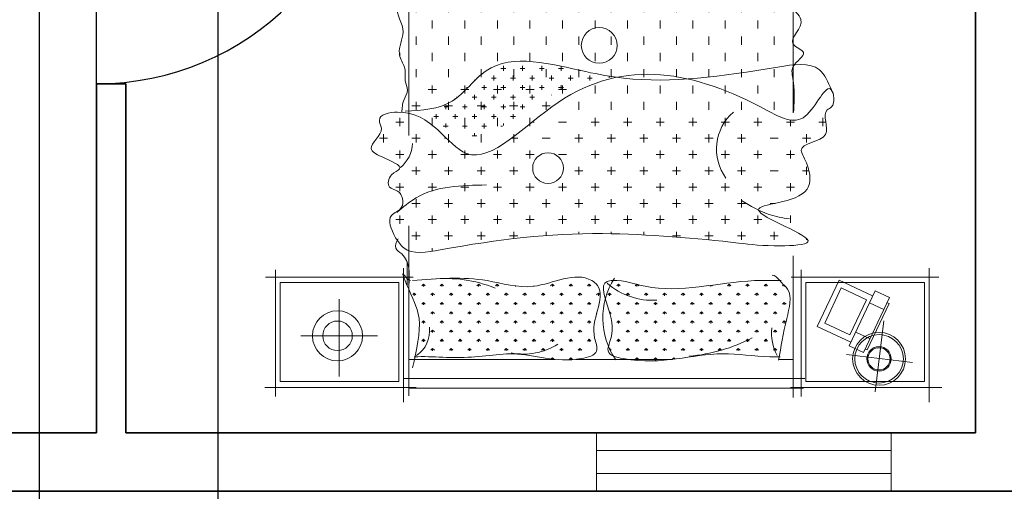
# Model space of a CAD drawing. Units: inches. Extents: x -26 to 575, y -18 to 513.
# Tile 3 of 28: x 122 to 274, y 119 to 191. Entities that reach past the tile are written whole.
import ezdxf

# ---------------------------------------------------------------- set-up
doc = ezdxf.new("R2010")
doc.units = ezdxf.units.IN
doc.header["$MEASUREMENT"] = 0
for name, color, linetype, lineweight in [('A-ANNO-DIMS', 2, 'Continuous', 18), ('A-DOOR', 3, 'Continuous', 25), ('A-GLAZ', 4, 'Continuous', 18), ('A-WALL', 7, 'Continuous', 35), ('Furniture', 8, 'Continuous', 15)]:
    doc.layers.add(name, color=color, linetype=linetype, lineweight=lineweight)
doc.styles.get("Standard").update_dxf_attribs({"font": 'arial.ttf', "height": 6})
doc.dimstyles.get("Standard").update_dxf_attribs({"dimtxt": 6, "dimasz": 0.18, "dimexe": 0.18, "dimexo": 0.0625, "dimgap": 0.09, "dimtad": 0, "dimtih": 1, "dimtoh": 1, "dimzin": 0, "dimdsep": 46, "dimlunit": 3, "dimtxsty": 'Standard', "dimcen": 0.09, "dimadec": 0, "dimazin": 0, "dimtfac": 1, "dimtofl": 0, "dimtmove": 0, "dimatfit": 3, "dimfxl": 1, "dimtolj": 1, "dimtzin": 0, "dimarcsym": 0})

# ---------------------------------------------------------------- blocks, each defined once
blk = doc.blocks.new('BED-DOUBLE-WITH-NIGHTSTANDS')
for p, q in [((1.93, 83.36), (1.93, 62.76)), ((82.67, 83.36), (82.67, 62.76)), ((10.27, 81.76), (8.94, 70.83)), ((21.61, 63.03), (21.61, 82.46)), ((22.83, 60.83), (22.83, 82.62)), ((81.88, 82.34), (81.88, 56.23)), ((102.35, 63.03), (102.35, 82.46)), ((23.23, 81.08), (0, 81.08)), ((20.89, 80.15), (2.67, 80.15)), ((2.67, 80.15), (2.67, 64.97)), ((20.89, 64.97), (20.89, 80.15)), ((21.24, 81.17), (81.88, 81.17)), ((103.97, 81.08), (80.74, 81.08)), ((101.63, 80.15), (83.41, 80.15)), ((83.41, 80.15), (83.41, 64.97)), ((101.63, 64.97), (101.63, 80.15)), ((82.67, 79.72), (21.06, 79.72)), ((92.57, 79.4), (92.57, 67.51)), ((14.67, 76.01), (4.51, 77.26)), ((8.06, 67.24), (12.03, 75.72)), ((12.03, 75.72), (14.23, 74.69)), ((25.06, 76.76), (22.83, 76.76)), ((41.17, 76.51), (40.96, 76.72)), ((41.17, 76.51), (41.43, 76.77)), ((41.17, 76.51), (41.17, 76.74)), ((56.23, 76.76), (41.36, 76.76)), ((44, 76.51), (43.73, 76.77)), ((44, 76.51), (44, 76.88)), ((44, 76.51), (44.26, 76.77)), ((46.83, 76.51), (46.56, 76.77)), ((46.83, 76.51), (46.83, 76.88)), ((46.83, 76.51), (47.09, 76.77)), ((57, 76.51), (56.74, 76.77)), ((57, 76.51), (57, 76.83)), ((57, 76.51), (57.27, 76.77)), ((81.88, 76.76), (59.39, 76.76)), ((59.83, 76.51), (59.59, 76.74)), ((59.83, 76.51), (59.83, 76.72)), ((59.83, 76.51), (60.02, 76.69)), ((11.46, 75.32), (8.12, 68.2)), ((14.23, 74.69), (10.26, 66.21)), ((11.77, 75.18), (11.46, 75.32)), ((19.14, 71.73), (13.98, 74.14)), ((25.61, 75.09), (25.35, 75.36)), ((25.61, 75.09), (25.61, 75.47)), ((25.61, 75.09), (25.88, 75.36)), ((28.44, 75.09), (28.18, 75.36)), ((28.44, 75.09), (28.44, 75.47)), ((28.44, 75.09), (28.71, 75.36)), ((31.27, 75.09), (31, 75.36)), ((31.27, 75.09), (31.27, 75.47)), ((31.27, 75.09), (31.53, 75.36)), ((34.1, 75.09), (33.83, 75.36)), ((34.1, 75.09), (34.1, 75.47)), ((34.1, 75.09), (34.36, 75.36)), ((36.93, 75.09), (36.66, 75.36)), ((36.93, 75.09), (36.93, 75.47)), ((36.93, 75.09), (37.19, 75.36)), ((39.75, 75.09), (39.49, 75.36)), ((39.75, 75.09), (39.75, 75.47)), ((39.75, 75.09), (40.02, 75.36)), ((42.58, 75.09), (42.32, 75.36)), ((42.58, 75.09), (42.58, 75.47)), ((42.58, 75.09), (42.85, 75.36)), ((45.41, 75.09), (45.15, 75.36)), ((45.41, 75.09), (45.41, 75.47)), ((45.41, 75.09), (45.68, 75.36)), ((48.24, 75.09), (47.97, 75.36)), ((48.24, 75.09), (48.24, 75.47)), ((48.24, 75.09), (48.5, 75.36)), ((51.07, 75.09), (50.8, 75.36)), ((51.07, 75.09), (51.07, 75.1)), ((51.07, 75.09), (51.07, 75.1)), ((53, 75.34), (53.03, 75.36)), ((55.59, 75.09), (55.32, 75.36)), ((55.59, 75.09), (55.59, 75.47)), ((55.59, 75.09), (55.85, 75.36)), ((58.42, 75.09), (58.15, 75.36)), ((58.42, 75.09), (58.42, 75.47)), ((58.42, 75.09), (58.68, 75.36)), ((61.25, 75.09), (60.98, 75.36)), ((61.25, 75.09), (61.25, 75.47)), ((61.25, 75.09), (61.51, 75.36)), ((64.07, 75.09), (63.81, 75.36)), ((64.07, 75.09), (64.07, 75.47)), ((64.07, 75.09), (64.34, 75.36)), ((66.9, 75.09), (66.64, 75.36)), ((66.9, 75.09), (66.9, 75.47)), ((66.9, 75.09), (67.17, 75.36)), ((69.73, 75.09), (69.47, 75.36)), ((69.73, 75.09), (69.73, 75.47)), ((69.73, 75.09), (70, 75.36)), ((72.56, 75.09), (72.29, 75.36)), ((72.56, 75.09), (72.56, 75.47)), ((72.56, 75.09), (72.82, 75.36)), ((75.39, 75.09), (75.12, 75.36)), ((75.39, 75.09), (75.39, 75.47)), ((75.39, 75.09), (75.65, 75.36)), ((78.22, 75.09), (77.95, 75.36)), ((78.22, 75.09), (78.22, 75.47)), ((78.22, 75.09), (78.48, 75.36)), ((13.24, 72.57), (11.03, 73.6)), ((14.13, 73), (11.6, 67.59)), ((17.98, 71.2), (14.13, 73)), ((25.61, 72.26), (25.61, 72.64)), ((27.03, 73.68), (26.76, 73.94)), ((27.03, 73.68), (27.03, 74.05)), ((27.03, 73.68), (27.29, 73.94)), ((28.44, 72.26), (28.44, 72.64)), ((29.85, 73.68), (29.59, 73.94)), ((29.85, 73.68), (30.12, 73.94)), ((29.86, 73.68), (29.86, 74.05)), ((31.27, 72.26), (31.27, 72.64)), ((32.68, 73.68), (32.42, 73.94)), ((32.68, 73.68), (32.68, 74.05)), ((32.68, 73.68), (32.95, 73.94)), ((34.1, 72.26), (34.1, 72.64)), ((35.51, 73.68), (35.25, 73.94)), ((35.51, 73.68), (35.51, 74.05)), ((35.51, 73.68), (35.78, 73.94)), ((36.93, 72.26), (36.93, 72.64)), ((38.34, 73.68), (38.07, 73.94)), ((38.34, 73.68), (38.34, 74.05)), ((38.34, 73.68), (38.61, 73.94)), ((39.75, 72.26), (39.75, 72.64)), ((41.17, 73.68), (40.9, 73.94)), ((41.17, 73.68), (41.17, 74.05)), ((41.17, 73.68), (41.43, 73.94)), ((42.58, 72.26), (42.58, 72.64)), ((44, 73.68), (43.73, 73.94)), ((44, 73.68), (44, 74.05)), ((44, 73.68), (44.26, 73.94)), ((45.41, 72.26), (45.41, 72.64)), ((46.83, 73.68), (46.56, 73.94)), ((46.83, 73.68), (46.83, 74.05)), ((46.83, 73.68), (47.09, 73.94)), ((48.24, 72.26), (48.24, 72.64)), ((49.65, 73.68), (49.39, 73.94)), ((49.65, 73.68), (49.65, 74.05)), ((49.65, 73.68), (49.92, 73.94)), ((54.17, 73.68), (53.91, 73.94)), ((54.17, 73.68), (54.17, 74.05)), ((54.17, 73.68), (54.44, 73.94)), ((55.59, 72.26), (55.59, 72.64)), ((57, 73.68), (56.74, 73.94)), ((57, 73.68), (57, 74.05)), ((57, 73.68), (57.27, 73.94)), ((58.42, 72.26), (58.42, 72.64)), ((59.83, 73.68), (59.57, 73.94)), ((59.83, 73.68), (59.83, 74.05)), ((59.83, 73.68), (60.1, 73.94)), ((61.25, 72.26), (61.25, 72.64)), ((62.66, 73.68), (62.39, 73.94)), ((62.66, 73.68), (62.66, 74.05)), ((62.66, 73.68), (62.92, 73.94)), ((64.07, 72.26), (64.07, 72.64)), ((65.49, 73.68), (65.22, 73.94)), ((65.49, 73.68), (65.49, 74.05)), ((65.49, 73.68), (65.75, 73.94)), ((66.9, 72.26), (66.9, 72.64)), ((68.32, 73.68), (68.05, 73.94)), ((68.32, 73.68), (68.32, 74.05)), ((68.32, 73.68), (68.58, 73.94)), ((69.73, 72.26), (69.73, 72.64)), ((71.14, 73.68), (70.88, 73.94)), ((71.14, 73.68), (71.41, 73.94)), ((71.15, 73.68), (71.15, 74.05)), ((72.56, 72.26), (72.56, 72.64)), ((73.97, 73.68), (73.71, 73.94)), ((73.97, 73.68), (73.97, 74.05)), ((73.97, 73.68), (74.24, 73.94)), ((75.39, 72.26), (75.39, 72.64)), ((76.8, 73.68), (76.54, 73.94)), ((76.8, 73.68), (76.8, 74.05)), ((76.8, 73.68), (77.07, 73.94)), ((78.22, 72.26), (78.22, 72.64)), ((79.63, 73.68), (79.36, 73.94)), ((79.63, 73.68), (79.63, 74.05)), ((79.63, 73.68), (79.9, 73.94)), ((98.47, 73.14), (86.67, 73.14)), ((15.45, 65.79), (17.98, 71.2)), ((15.8, 64.6), (19.14, 71.73)), ((24.2, 70.85), (23.97, 71.08)), ((24.2, 70.85), (24.2, 71.23)), ((24.2, 70.85), (24.46, 71.12)), ((25.61, 72.26), (25.35, 72.53)), ((25.61, 72.26), (25.88, 72.53)), ((27.03, 70.85), (26.76, 71.12)), ((27.03, 70.85), (27.03, 71.23)), ((27.03, 70.85), (27.29, 71.12)), ((28.44, 72.26), (28.18, 72.53)), ((28.44, 72.26), (28.71, 72.53)), ((29.85, 70.85), (29.59, 71.12)), ((29.85, 70.85), (30.12, 71.12)), ((29.86, 70.85), (29.86, 71.23)), ((31.27, 72.26), (31, 72.53)), ((31.27, 72.26), (31.53, 72.53)), ((32.68, 70.85), (32.42, 71.12)), ((32.68, 70.85), (32.68, 71.23)), ((32.68, 70.85), (32.95, 71.12)), ((34.1, 72.26), (33.83, 72.53)), ((34.1, 72.26), (34.36, 72.53)), ((35.51, 70.85), (35.25, 71.12)), ((35.51, 70.85), (35.51, 71.23)), ((35.51, 70.85), (35.78, 71.12)), ((36.93, 72.26), (36.66, 72.53)), ((36.93, 72.26), (37.19, 72.53)), ((38.34, 70.85), (38.07, 71.12)), ((38.34, 70.85), (38.34, 71.23)), ((38.34, 70.85), (38.61, 71.12)), ((39.75, 72.26), (39.49, 72.53)), ((39.75, 72.26), (40.02, 72.53)), ((41.17, 70.85), (40.9, 71.12)), ((41.17, 70.85), (41.17, 71.23)), ((41.17, 70.85), (41.43, 71.12)), ((42.58, 72.26), (42.32, 72.53)), ((42.58, 72.26), (42.85, 72.53)), ((44, 70.85), (43.73, 71.12)), ((44, 70.85), (44, 71.23)), ((44, 70.85), (44.26, 71.12)), ((45.41, 72.26), (45.15, 72.53)), ((45.41, 72.26), (45.68, 72.53)), ((46.83, 70.85), (46.56, 71.12)), ((46.83, 70.85), (46.83, 71.23)), ((46.83, 70.85), (47.09, 71.12)), ((48.24, 72.26), (47.97, 72.53)), ((48.24, 72.26), (48.5, 72.53)), ((49.65, 70.85), (49.39, 71.12)), ((49.65, 70.85), (49.65, 71.23)), ((49.65, 70.85), (49.92, 71.12)), ((54.17, 70.85), (53.91, 71.12)), ((54.17, 70.85), (54.17, 71.23)), ((54.17, 70.85), (54.44, 71.12)), ((55.59, 72.26), (55.32, 72.53)), ((55.59, 72.26), (55.85, 72.53)), ((57, 70.85), (56.74, 71.12)), ((57, 70.85), (57, 71.23)), ((57, 70.85), (57.27, 71.12)), ((58.42, 72.26), (58.15, 72.53)), ((58.42, 72.26), (58.68, 72.53)), ((59.83, 70.85), (59.57, 71.12)), ((59.83, 70.85), (59.83, 71.23)), ((59.83, 70.85), (60.1, 71.12)), ((61.25, 72.26), (60.98, 72.53)), ((61.25, 72.26), (61.51, 72.53)), ((62.66, 70.85), (62.39, 71.12)), ((62.66, 70.85), (62.66, 71.23)), ((62.66, 70.85), (62.92, 71.12)), ((64.07, 72.26), (63.81, 72.53)), ((64.07, 72.26), (64.34, 72.53)), ((65.49, 70.85), (65.22, 71.12)), ((65.49, 70.85), (65.49, 71.23)), ((65.49, 70.85), (65.75, 71.12)), ((66.9, 72.26), (66.64, 72.53)), ((66.9, 72.26), (67.17, 72.53)), ((68.32, 70.85), (68.05, 71.12)), ((68.32, 70.85), (68.32, 71.23)), ((68.32, 70.85), (68.58, 71.12)), ((69.73, 72.26), (69.47, 72.53)), ((69.73, 72.26), (70, 72.53)), ((71.14, 70.85), (70.88, 71.12)), ((71.14, 70.85), (71.41, 71.12)), ((71.15, 70.85), (71.15, 71.23)), ((72.56, 72.26), (72.29, 72.53)), ((72.56, 72.26), (72.82, 72.53)), ((73.97, 70.85), (73.71, 71.12)), ((73.97, 70.85), (73.97, 71.23)), ((73.97, 70.85), (74.24, 71.12)), ((75.39, 72.26), (75.12, 72.53)), ((75.39, 72.26), (75.65, 72.53)), ((76.8, 70.85), (76.54, 71.12)), ((76.8, 70.85), (76.8, 71.23)), ((76.8, 70.85), (77.07, 71.12)), ((78.22, 72.26), (77.95, 72.53)), ((78.22, 72.26), (78.48, 72.53)), ((79.63, 70.85), (79.36, 71.12)), ((79.63, 70.85), (79.63, 71.23)), ((79.63, 70.85), (79.9, 71.12)), ((25.61, 69.44), (25.35, 69.7)), ((25.61, 69.44), (25.61, 69.81)), ((25.61, 69.44), (25.88, 69.7)), ((28.44, 69.44), (28.18, 69.7)), ((28.44, 69.44), (28.44, 69.81)), ((28.44, 69.44), (28.71, 69.7)), ((31.27, 69.44), (31, 69.7)), ((31.27, 69.44), (31.27, 69.81)), ((31.27, 69.44), (31.53, 69.7)), ((34.1, 69.44), (33.83, 69.7)), ((34.1, 69.44), (34.1, 69.81)), ((34.1, 69.44), (34.36, 69.7)), ((36.93, 69.44), (36.66, 69.7)), ((36.93, 69.44), (36.93, 69.81)), ((36.93, 69.44), (37.19, 69.7)), ((39.75, 69.44), (39.49, 69.7)), ((39.75, 69.44), (39.75, 69.81)), ((39.75, 69.44), (40.02, 69.7)), ((42.58, 69.44), (42.32, 69.7)), ((42.58, 69.44), (42.58, 69.81)), ((42.58, 69.44), (42.85, 69.7)), ((45.41, 69.44), (45.15, 69.7)), ((45.41, 69.44), (45.41, 69.81)), ((45.41, 69.44), (45.68, 69.7)), ((48.24, 69.44), (47.97, 69.7)), ((48.24, 69.44), (48.24, 69.81)), ((48.24, 69.44), (48.5, 69.7)), ((51.05, 69.45), (50.8, 69.7)), ((53.01, 69.68), (53.03, 69.7)), ((55.59, 69.44), (55.32, 69.7)), ((55.59, 69.44), (55.59, 69.81)), ((55.59, 69.44), (55.85, 69.7)), ((58.42, 69.44), (58.15, 69.7)), ((58.42, 69.44), (58.42, 69.81)), ((58.42, 69.44), (58.68, 69.7)), ((61.25, 69.44), (60.98, 69.7)), ((61.25, 69.44), (61.25, 69.81)), ((61.25, 69.44), (61.51, 69.7)), ((64.07, 69.44), (63.81, 69.7)), ((64.07, 69.44), (64.07, 69.81)), ((64.07, 69.44), (64.34, 69.7)), ((66.9, 69.44), (66.64, 69.7)), ((66.9, 69.44), (66.9, 69.81)), ((66.9, 69.44), (67.17, 69.7)), ((69.73, 69.44), (69.47, 69.7)), ((69.73, 69.44), (69.73, 69.81)), ((69.73, 69.44), (70, 69.7)), ((72.56, 69.44), (72.29, 69.7)), ((72.56, 69.44), (72.56, 69.81)), ((72.56, 69.44), (72.82, 69.7)), ((75.39, 69.44), (75.12, 69.7)), ((75.39, 69.44), (75.39, 69.81)), ((75.39, 69.44), (75.65, 69.7)), ((78.22, 69.44), (77.95, 69.7)), ((78.22, 69.44), (78.22, 69.81)), ((78.22, 69.44), (78.48, 69.7)), ((8.12, 68.2), (8.43, 68.05)), ((11.14, 68.07), (8.93, 69.1)), ((24.2, 68.02), (23.93, 68.29)), ((24.2, 68.02), (24.2, 68.4)), ((24.2, 68.02), (24.46, 68.29)), ((27.03, 68.02), (26.76, 68.29)), ((27.03, 68.02), (27.03, 68.4)), ((27.03, 68.02), (27.29, 68.29)), ((29.85, 68.02), (29.59, 68.29)), ((29.85, 68.02), (30.12, 68.29)), ((29.86, 68.02), (29.86, 68.4)), ((32.68, 68.02), (32.42, 68.29)), ((32.68, 68.02), (32.68, 68.4)), ((32.68, 68.02), (32.95, 68.29)), ((35.51, 68.02), (35.25, 68.29)), ((35.51, 68.02), (35.51, 68.4)), ((35.51, 68.02), (35.78, 68.29)), ((38.34, 68.02), (38.07, 68.29)), ((38.34, 68.02), (38.34, 68.4)), ((38.34, 68.02), (38.61, 68.29)), ((41.17, 68.02), (40.9, 68.29)), ((41.17, 68.02), (41.17, 68.4)), ((41.17, 68.02), (41.43, 68.29)), ((44, 68.02), (43.73, 68.29)), ((44, 68.02), (44, 68.4)), ((44, 68.02), (44.26, 68.29)), ((46.83, 68.02), (46.56, 68.29)), ((46.83, 68.02), (46.83, 68.4)), ((46.83, 68.02), (47.09, 68.29)), ((49.65, 68.02), (49.39, 68.29)), ((49.65, 68.02), (49.65, 68.4)), ((49.65, 68.02), (49.92, 68.29)), ((54.17, 68.02), (53.91, 68.29)), ((54.17, 68.02), (54.17, 68.4)), ((54.17, 68.02), (54.44, 68.29)), ((57, 68.02), (56.74, 68.29)), ((57, 68.02), (57, 68.4)), ((57, 68.02), (57.27, 68.29)), ((59.83, 68.02), (59.57, 68.29)), ((59.83, 68.02), (59.83, 68.4)), ((59.83, 68.02), (60.1, 68.29)), ((62.66, 68.02), (62.39, 68.29)), ((62.66, 68.02), (62.66, 68.4)), ((62.66, 68.02), (62.92, 68.29)), ((65.49, 68.02), (65.22, 68.29)), ((65.49, 68.02), (65.49, 68.4)), ((65.49, 68.02), (65.75, 68.29)), ((68.32, 68.02), (68.05, 68.29)), ((68.32, 68.02), (68.32, 68.4)), ((68.32, 68.02), (68.58, 68.29)), ((71.14, 68.02), (70.88, 68.29)), ((71.14, 68.02), (71.41, 68.29)), ((71.15, 68.02), (71.15, 68.4)), ((73.97, 68.02), (73.71, 68.29)), ((73.97, 68.02), (73.97, 68.4)), ((73.97, 68.02), (74.24, 68.29)), ((76.8, 68.02), (76.54, 68.29)), ((76.8, 68.02), (76.8, 68.4)), ((76.8, 68.02), (77.07, 68.29)), ((79.63, 68.02), (79.36, 68.29)), ((79.63, 68.02), (79.63, 68.4)), ((79.63, 68.02), (79.9, 68.29)), ((10.26, 66.21), (8.06, 67.24)), ((10.64, 67.02), (15.8, 64.6)), ((11.6, 67.59), (15.45, 65.79)), ((25.61, 66.61), (25.35, 66.87)), ((25.61, 66.61), (25.61, 66.98)), ((25.61, 66.61), (25.88, 66.87)), ((28.44, 66.61), (28.18, 66.87)), ((28.44, 66.61), (28.44, 66.98)), ((28.44, 66.61), (28.71, 66.87)), ((31.27, 66.61), (31, 66.87)), ((31.27, 66.61), (31.27, 66.98)), ((31.27, 66.61), (31.53, 66.87)), ((34.1, 66.61), (33.83, 66.87)), ((34.1, 66.61), (34.1, 66.98)), ((34.1, 66.61), (34.36, 66.87)), ((36.93, 66.61), (36.66, 66.87)), ((36.93, 66.61), (36.93, 66.98)), ((36.93, 66.61), (37.19, 66.87)), ((39.75, 66.61), (39.49, 66.87)), ((39.75, 66.61), (39.75, 66.98)), ((39.75, 66.61), (40.02, 66.87)), ((42.58, 66.61), (42.32, 66.87)), ((42.58, 66.61), (42.58, 66.98)), ((42.58, 66.61), (42.85, 66.87)), ((45.41, 66.61), (45.15, 66.87)), ((45.41, 66.61), (45.41, 66.98)), ((45.41, 66.61), (45.68, 66.87)), ((48.24, 66.61), (47.97, 66.87)), ((48.24, 66.61), (48.24, 66.98)), ((48.24, 66.61), (48.5, 66.87)), ((51.07, 66.61), (50.8, 66.87)), ((51.07, 66.61), (51.07, 66.98)), ((51.07, 66.61), (51.33, 66.87)), ((52.76, 66.61), (52.49, 66.87)), ((52.76, 66.61), (52.76, 66.98)), ((52.76, 66.61), (53.03, 66.87)), ((55.59, 66.61), (55.32, 66.87)), ((55.59, 66.61), (55.59, 66.98)), ((55.59, 66.61), (55.85, 66.87)), ((58.42, 66.61), (58.15, 66.87)), ((58.42, 66.61), (58.42, 66.98)), ((58.42, 66.61), (58.68, 66.87)), ((61.25, 66.61), (60.98, 66.87)), ((61.25, 66.61), (61.25, 66.98)), ((61.25, 66.61), (61.51, 66.87)), ((64.07, 66.61), (63.81, 66.87)), ((64.07, 66.61), (64.07, 66.98)), ((64.07, 66.61), (64.34, 66.87)), ((66.9, 66.61), (66.64, 66.87)), ((66.9, 66.61), (66.9, 66.98)), ((66.9, 66.61), (67.17, 66.87)), ((69.73, 66.61), (69.47, 66.87)), ((69.73, 66.61), (69.73, 66.98)), ((69.73, 66.61), (70, 66.87)), ((72.56, 66.61), (72.29, 66.87)), ((72.56, 66.61), (72.56, 66.98)), ((72.56, 66.61), (72.82, 66.87)), ((75.39, 66.61), (75.12, 66.87)), ((75.39, 66.61), (75.39, 66.98)), ((75.39, 66.61), (75.65, 66.87)), ((78.22, 66.61), (77.95, 66.87)), ((78.22, 66.61), (78.22, 66.98)), ((78.22, 66.61), (78.48, 66.87)), ((81.04, 66.61), (80.78, 66.87)), ((81.04, 66.61), (81.04, 66.98)), ((81.04, 66.61), (81.25, 66.82)), ((24.2, 65.39), (24.2, 65.57)), ((24.29, 65.29), (24.46, 65.46)), ((27.03, 65.19), (26.76, 65.46)), ((27.03, 65.19), (27.03, 65.57)), ((27.03, 65.19), (27.29, 65.46)), ((29.85, 65.19), (29.59, 65.46)), ((29.85, 65.19), (30.12, 65.46)), ((29.86, 65.19), (29.86, 65.57)), ((32.68, 65.19), (32.42, 65.46)), ((32.68, 65.19), (32.68, 65.57)), ((32.68, 65.19), (32.95, 65.46)), ((35.33, 65.37), (35.25, 65.46)), ((35.51, 65.39), (35.51, 65.57)), ((35.74, 65.42), (35.78, 65.46)), ((46.77, 65.25), (46.56, 65.46)), ((46.83, 65.23), (46.83, 65.57)), ((46.86, 65.22), (47.09, 65.46)), ((49.65, 65.19), (49.39, 65.46)), ((49.65, 65.19), (49.65, 65.57)), ((49.65, 65.19), (49.92, 65.46)), ((54.17, 65.19), (53.91, 65.46)), ((54.17, 65.19), (54.17, 65.57)), ((54.17, 65.19), (54.44, 65.46)), ((57, 65.19), (56.74, 65.46)), ((57, 65.19), (57, 65.57)), ((57, 65.19), (57.27, 65.46)), ((59.83, 65.19), (59.57, 65.46)), ((59.83, 65.19), (59.83, 65.57)), ((59.83, 65.19), (60.1, 65.46)), ((62.66, 65.52), (62.66, 65.57)), ((65.49, 65.48), (65.49, 65.57)), ((65.74, 65.45), (65.75, 65.46)), ((68.32, 65.19), (68.05, 65.46)), ((68.32, 65.19), (68.32, 65.57)), ((68.32, 65.19), (68.58, 65.46)), ((71.14, 65.19), (70.88, 65.46)), ((71.14, 65.19), (71.41, 65.46)), ((71.15, 65.19), (71.15, 65.57)), ((73.97, 65.19), (73.71, 65.46)), ((73.97, 65.19), (73.97, 65.57)), ((73.97, 65.19), (74.24, 65.46)), ((76.8, 65.19), (76.54, 65.46)), ((76.8, 65.19), (76.8, 65.57)), ((76.8, 65.19), (77.07, 65.46)), ((79.63, 65.19), (79.36, 65.46)), ((79.63, 65.19), (79.63, 65.57)), ((79.63, 65.19), (79.9, 65.46)), ((82.15, 61.74), (82.15, 65.42)), ((0.45, 64.15), (23.14, 64.15)), ((2.67, 64.97), (20.89, 64.97)), ((55.59, 64.12), (55.59, 64.15)), ((81.19, 64.15), (103.88, 64.15)), ((83.41, 64.97), (101.63, 64.97)), ((78.27, 59.67), (78.27, 60.15)), ((20.77, 58.21), (20.77, 58.42)), ((21.39, 57.79), (21.31, 57.79)), ((26.39, 57.79), (25.14, 57.79)), ((25.77, 57.17), (25.77, 58.42)), ((31.39, 57.79), (30.14, 57.79)), ((30.77, 57.17), (30.77, 58.42)), ((36.39, 57.79), (35.14, 57.79)), ((35.77, 57.17), (35.77, 58.41)), ((41.39, 57.79), (40.14, 57.79)), ((40.77, 57.17), (40.77, 57.97)), ((45.77, 57.17), (45.77, 57.64)), ((55.77, 57.17), (55.77, 57.48)), ((60.77, 57.17), (60.77, 57.74)), ((66.39, 57.79), (65.14, 57.79)), ((65.77, 57.17), (65.77, 58.21)), ((71.39, 57.79), (70.14, 57.79)), ((70.77, 57.17), (70.77, 58.42)), ((76.39, 57.79), (75.14, 57.79)), ((75.77, 57.17), (75.77, 58.42)), ((81.39, 57.79), (80.14, 57.79)), ((80.77, 57.17), (80.77, 58.42)), ((50.77, 57.17), (50.77, 57.46)), ((23.27, 54.64), (23.27, 55.76)), ((28.89, 55.29), (27.64, 55.29)), ((28.27, 54.67), (28.27, 55.92)), ((33.89, 55.29), (32.64, 55.29)), ((33.27, 54.67), (33.27, 55.92)), ((38.89, 55.29), (37.64, 55.29)), ((38.27, 54.67), (38.27, 55.92)), ((43.89, 55.29), (42.64, 55.29)), ((43.27, 54.67), (43.27, 55.92)), ((48.89, 55.29), (47.64, 55.29)), ((48.27, 54.67), (48.27, 55.92)), ((53.89, 55.29), (52.64, 55.29)), ((53.27, 54.67), (53.27, 55.92)), ((58.89, 55.29), (57.64, 55.29)), ((58.27, 54.67), (58.27, 55.92)), ((63.89, 55.29), (62.64, 55.29)), ((63.27, 54.67), (63.27, 55.92)), ((68.89, 55.29), (67.64, 55.29)), ((68.27, 54.67), (68.27, 55.92)), ((73.89, 55.29), (72.64, 55.29)), ((73.27, 54.67), (73.27, 55.92)), ((78.89, 55.29), (77.64, 55.29)), ((78.27, 54.67), (78.27, 55.92)), ((83.89, 55.29), (82.64, 55.29)), ((83.27, 54.67), (83.27, 55.92)), ((30.77, 52.17), (30.77, 53.42)), ((35.77, 52.17), (35.77, 53.42)), ((40.77, 52.17), (40.77, 53.42)), ((45.77, 52.17), (45.77, 53.42)), ((50.77, 52.17), (50.77, 53.42)), ((55.77, 52.17), (55.77, 53.42)), ((60.77, 52.17), (60.77, 53.42)), ((65.77, 52.17), (65.77, 53.42)), ((70.77, 52.17), (70.77, 53.42)), ((75.77, 52.17), (75.77, 53.42)), ((80.77, 52.17), (80.77, 53.42)), ((26.39, 52.79), (25.62, 52.79)), ((31.39, 52.79), (30.14, 52.79)), ((36.39, 52.79), (35.14, 52.79)), ((41.39, 52.79), (40.14, 52.79)), ((46.39, 52.79), (45.14, 52.79)), ((51.39, 52.79), (50.14, 52.79)), ((56.39, 52.79), (55.14, 52.79)), ((61.39, 52.79), (60.14, 52.79)), ((66.39, 52.79), (65.14, 52.79)), ((71.39, 52.79), (70.14, 52.79)), ((76.39, 52.79), (75.14, 52.79)), ((81.39, 52.79), (80.14, 52.79)), ((23.89, 50.29), (22.64, 50.29)), ((23.27, 49.67), (23.27, 50.92)), ((28.89, 50.29), (27.64, 50.29)), ((28.27, 49.67), (28.27, 50.92)), ((33.89, 50.29), (32.64, 50.29)), ((33.27, 49.67), (33.27, 50.92)), ((38.89, 50.29), (37.64, 50.29)), ((38.27, 49.67), (38.27, 50.92)), ((43.89, 50.29), (42.64, 50.29)), ((43.27, 49.67), (43.27, 50.92)), ((48.89, 50.29), (47.64, 50.29)), ((48.27, 49.67), (48.27, 50.92)), ((53.89, 50.29), (52.64, 50.29)), ((53.27, 49.67), (53.27, 50.92)), ((58.89, 50.29), (57.64, 50.29)), ((58.27, 49.67), (58.27, 50.92)), ((63.89, 50.29), (62.64, 50.29)), ((63.27, 49.67), (63.27, 50.92)), ((68.89, 50.29), (67.64, 50.29)), ((68.27, 49.67), (68.27, 50.92)), ((73.89, 50.29), (72.64, 50.29)), ((73.27, 49.67), (73.27, 50.92)), ((78.89, 50.29), (77.64, 50.29)), ((78.27, 49.67), (78.27, 50.92)), ((83.89, 50.29), (82.64, 50.29)), ((83.27, 49.67), (83.27, 50.92)), ((20.77, 47.17), (20.77, 48.42)), ((30.77, 47.17), (30.77, 48.42)), ((35.77, 47.17), (35.77, 48.42)), ((40.77, 47.17), (40.77, 48.42)), ((45.77, 47.17), (45.77, 48.42)), ((50.77, 47.17), (50.77, 48.42)), ((55.77, 47.17), (55.77, 48.42)), ((65.77, 47.17), (65.77, 48.42)), ((70.77, 47.17), (70.77, 48.42)), ((75.77, 47.17), (75.77, 48.42)), ((80.77, 47.17), (80.77, 48.42)), ((21.39, 47.79), (20.41, 47.79)), ((26.39, 47.79), (25.14, 47.79)), ((31.39, 47.79), (30.14, 47.79)), ((36.39, 47.79), (35.14, 47.79)), ((41.39, 47.79), (40.14, 47.79)), ((46.39, 47.79), (45.14, 47.79)), ((51.39, 47.79), (50.14, 47.79)), ((56.39, 47.79), (55.14, 47.79)), ((66.39, 47.79), (65.14, 47.79)), ((71.39, 47.79), (70.14, 47.79)), ((76.39, 47.79), (75.14, 47.79)), ((81.39, 47.79), (80.14, 47.79)), ((23.27, 44.67), (23.27, 45.92)), ((28.27, 44.67), (28.27, 45.92)), ((33.27, 44.67), (33.27, 45.92)), ((38.27, 44.67), (38.27, 45.92)), ((43.27, 44.67), (43.27, 45.92)), ((48.27, 44.67), (48.27, 45.92)), ((53.27, 44.67), (53.27, 45.92)), ((63.27, 44.67), (63.27, 45.92)), ((68.27, 44.67), (68.27, 45.92)), ((73.27, 44.67), (73.27, 45.92)), ((78.27, 44.67), (78.27, 45.92)), ((83.27, 44.67), (83.27, 45.92)), ((23.89, 45.29), (22.64, 45.29)), ((28.89, 45.29), (27.64, 45.29)), ((33.89, 45.29), (32.64, 45.29)), ((38.89, 45.29), (37.64, 45.29)), ((43.89, 45.29), (42.64, 45.29)), ((48.89, 45.29), (47.64, 45.29)), ((53.89, 45.29), (52.64, 45.29)), ((58.89, 45.29), (57.64, 45.29)), ((63.89, 45.29), (62.64, 45.29)), ((68.89, 45.29), (67.64, 45.29)), ((73.89, 45.29), (72.64, 45.29)), ((78.89, 45.29), (77.64, 45.29)), ((83.89, 45.29), (82.64, 45.29)), ((21.39, 42.79), (20.14, 42.79)), ((20.77, 42.17), (20.77, 43.42)), ((26.39, 42.79), (25.14, 42.79)), ((31.39, 42.79), (30.14, 42.79)), ((30.77, 42.17), (30.77, 43.42)), ((36.39, 42.79), (35.14, 42.79)), ((35.77, 42.17), (35.77, 43.42)), ((41.39, 42.79), (40.14, 42.79)), ((40.77, 42.17), (40.77, 43.42)), ((46.39, 42.79), (45.14, 42.79)), ((45.77, 42.17), (45.77, 43.42)), ((51.39, 42.79), (50.14, 42.79)), ((50.77, 42.17), (50.77, 43.42)), ((56.39, 42.79), (55.14, 42.79)), ((55.77, 42.17), (55.77, 43.42)), ((61.39, 42.79), (60.14, 42.79)), ((66.09, 42.79), (65.14, 42.79)), ((65.77, 42.17), (65.77, 43.42)), ((70.77, 42.17), (70.77, 43.42)), ((72.15, 42.39), (71.41, 42.39)), ((71.78, 42.02), (71.78, 42.49)), ((75.77, 42.17), (75.77, 43.42)), ((76.39, 42.79), (76.07, 42.79)), ((81.39, 42.79), (80.14, 42.79)), ((80.77, 42.17), (80.77, 43.42)), ((81.88, 42.36), (81.88, 0)), ((86.39, 42.79), (85.14, 42.79)), ((85.77, 42.17), (85.77, 43.42)), ((18.27, 39.67), (18.27, 40.92)), ((23.27, 39.99), (23.27, 40.92)), ((28.27, 39.67), (28.27, 40.92)), ((33.27, 39.67), (33.27, 40.92)), ((38.27, 39.67), (38.27, 40.92)), ((43.27, 39.67), (43.27, 40.92)), ((48.27, 39.67), (48.27, 40.92)), ((53.27, 39.67), (53.27, 40.92)), ((63.27, 39.67), (63.27, 40.92)), ((67.35, 40.54), (67.35, 40.84)), ((67.72, 40.91), (67.48, 40.91)), ((68.27, 39.67), (68.27, 40.92)), ((70.67, 40.91), (69.93, 40.91)), ((70.3, 40.54), (70.3, 41.28)), ((73.62, 40.91), (72.89, 40.91)), ((73.26, 40.54), (73.26, 41.28)), ((73.27, 39.67), (73.27, 40.92)), ((76.58, 40.91), (75.84, 40.91)), ((76.21, 40.54), (76.21, 41.13)), ((78.27, 39.67), (78.27, 40.92)), ((83.27, 39.67), (83.27, 40.92)), ((18.89, 40.29), (17.83, 40.29)), ((23.89, 40.29), (22.64, 40.29)), ((28.89, 40.29), (27.64, 40.29)), ((33.89, 40.29), (32.64, 40.29)), ((38.89, 40.29), (37.64, 40.29)), ((43.89, 40.29), (42.64, 40.29)), ((48.89, 40.29), (47.64, 40.29)), ((53.89, 40.29), (52.64, 40.29)), ((58.89, 40.29), (57.64, 40.29)), ((62.9, 40.29), (62.64, 40.29)), ((66.24, 39.43), (65.5, 39.43)), ((65.87, 39.06), (65.87, 39.8)), ((69.2, 39.43), (68.46, 39.43)), ((68.83, 39.06), (68.83, 39.8)), ((72.15, 39.43), (71.41, 39.43)), ((71.78, 39.06), (71.78, 39.8)), ((75.1, 39.43), (74.36, 39.43)), ((74.73, 39.06), (74.73, 39.8)), ((78.05, 39.43), (77.32, 39.43)), ((77.68, 39.06), (77.68, 39.8)), ((83.89, 40.29), (82.64, 40.29)), ((22.83, 3.42), (22.83, 38.86)), ((25.77, 37.17), (25.77, 38.42)), ((30.77, 37.17), (30.77, 38.42)), ((35.77, 37.17), (35.77, 38.42)), ((40.77, 37.17), (40.77, 38.42)), ((45.77, 37.17), (45.77, 38.42)), ((50.77, 37.17), (50.77, 38.42)), ((55.77, 37.17), (55.77, 38.42)), ((60.77, 37.17), (60.77, 38.42)), ((64.77, 37.96), (64.03, 37.96)), ((64.4, 37.59), (64.4, 38.33)), ((65.77, 37.17), (65.77, 38.42)), ((67.72, 37.96), (66.98, 37.96)), ((67.35, 37.59), (67.35, 38.33)), ((70.67, 37.96), (69.93, 37.96)), ((70.3, 37.59), (70.3, 38.33)), ((70.77, 37.17), (70.77, 38.42)), ((73.62, 37.96), (72.89, 37.96)), ((73.26, 37.59), (73.26, 38.33)), ((75.77, 37.17), (75.77, 38.42)), ((76.45, 37.96), (75.84, 37.96)), ((76.21, 37.8), (76.21, 38.33)), ((80.77, 37.17), (80.77, 38.42)), ((61.39, 37.79), (60.14, 37.79)), ((63.29, 36.48), (62.55, 36.48)), ((62.92, 36.11), (62.92, 36.85)), ((66.39, 37.79), (65.14, 37.79)), ((66.24, 36.48), (65.5, 36.48)), ((65.87, 36.11), (65.87, 36.85)), ((69.2, 36.48), (68.46, 36.48)), ((68.83, 36.11), (68.83, 36.85)), ((71.39, 37.79), (70.14, 37.79)), ((72.15, 36.48), (71.41, 36.48)), ((71.78, 36.11), (71.78, 36.85)), ((74.53, 36.48), (74.36, 36.48)), ((74.73, 36.66), (74.73, 36.85)), ((76.39, 37.79), (75.14, 37.79)), ((81.39, 37.79), (80.14, 37.79)), ((17.66, 35.29), (17.64, 35.29)), ((28.27, 34.67), (28.27, 35.92)), ((33.27, 34.67), (33.27, 35.92)), ((38.27, 34.67), (38.27, 35.92)), ((43.27, 34.67), (43.27, 35.92)), ((48.27, 34.67), (48.27, 35.92)), ((53.27, 34.67), (53.27, 35.92)), ((58.89, 35.29), (57.64, 35.29)), ((58.86, 35), (58.12, 35)), ((58.27, 34.67), (58.27, 35.92)), ((58.49, 34.64), (58.49, 35.37)), ((59.97, 36.11), (59.97, 36.16)), ((61.81, 35), (61.08, 35)), ((61.44, 34.64), (61.44, 35.37)), ((63.89, 35.29), (62.64, 35.29)), ((63.27, 34.67), (63.27, 35.92)), ((64.77, 35), (64.03, 35)), ((64.4, 34.64), (64.4, 35.37)), ((67.72, 35), (66.98, 35)), ((67.35, 34.64), (67.35, 35.37)), ((68.89, 35.29), (67.64, 35.29)), ((68.27, 34.67), (68.27, 35.92)), ((70.67, 35), (69.93, 35)), ((70.3, 34.64), (70.3, 35.37)), ((73.89, 35.29), (72.64, 35.29)), ((73.01, 35), (72.89, 35)), ((73.26, 35.25), (73.26, 35.37)), ((73.27, 34.67), (73.27, 35.92)), ((78.89, 35.29), (77.64, 35.29)), ((78.27, 34.67), (78.27, 35.92)), ((25.77, 32.17), (25.77, 33.42)), ((30.77, 32.17), (30.77, 33.42)), ((35.77, 32.17), (35.77, 33.42)), ((40.77, 32.17), (40.77, 33.42)), ((45.77, 32.17), (45.77, 33.42)), ((50.77, 32.17), (50.77, 33.42)), ((51.11, 33.25), (51.11, 33.48)), ((54.43, 33.53), (53.69, 33.53)), ((54.06, 33.16), (54.06, 33.9)), ((55.77, 32.17), (55.77, 33.42)), ((57.38, 33.53), (56.65, 33.53)), ((57.02, 33.16), (57.02, 33.9)), ((60.34, 33.53), (59.6, 33.53)), ((59.97, 33.16), (59.97, 33.9)), ((60.77, 32.17), (60.77, 33.42)), ((63.29, 33.53), (62.55, 33.53)), ((62.92, 33.16), (62.92, 33.9)), ((66.24, 33.53), (65.5, 33.53)), ((65.77, 32.17), (65.77, 33.42)), ((65.87, 33.16), (65.87, 33.9)), ((69.2, 33.53), (68.46, 33.53)), ((68.83, 33.16), (68.83, 33.9)), ((70.77, 32.17), (70.77, 33.42)), ((71.47, 33.53), (71.41, 33.53)), ((71.78, 33.81), (71.78, 33.9)), ((75.77, 32.17), (75.77, 33.42)), ((80.77, 32.17), (80.77, 33.42)), ((55.54, 32.37), (55.54, 32.42)), ((58.86, 32.05), (58.12, 32.05)), ((58.49, 31.74), (58.49, 32.42)), ((61.81, 32.05), (61.08, 32.05)), ((61.44, 31.68), (61.44, 32.42)), ((64.77, 32.05), (64.03, 32.05)), ((64.4, 31.68), (64.4, 32.42)), ((67.72, 32.05), (66.98, 32.05)), ((67.35, 31.68), (67.35, 32.42)), ((28.27, 29.67), (28.27, 30.92)), ((33.27, 29.67), (33.27, 30.92)), ((38.27, 29.67), (38.27, 30.92)), ((43.27, 29.67), (43.27, 30.92)), ((48.27, 29.67), (48.27, 30.92)), ((53.27, 29.67), (53.27, 30.92)), ((58.27, 29.67), (58.27, 30.92)), ((63.27, 29.67), (63.27, 30.92)), ((68.27, 29.67), (68.27, 30.92)), ((73.27, 29.67), (73.27, 30.92)), ((78.27, 29.67), (78.27, 30.92)), ((83.27, 29.67), (83.27, 30.11)), ((25.77, 27.17), (25.77, 28.42)), ((30.77, 27.17), (30.77, 28.42)), ((35.77, 27.17), (35.77, 28.42)), ((40.77, 27.17), (40.77, 28.42)), ((45.77, 27.17), (45.77, 28.42)), ((50.77, 27.17), (50.77, 28.42)), ((55.77, 27.17), (55.77, 28.42)), ((60.77, 27.17), (60.77, 28.42)), ((65.77, 27.17), (65.77, 28.42)), ((70.77, 27.17), (70.77, 28.42)), ((75.77, 27.17), (75.77, 28.42)), ((80.77, 27.17), (80.77, 28.42)), ((28.27, 24.67), (28.27, 25.92)), ((33.27, 24.67), (33.27, 25.92)), ((38.27, 24.67), (38.27, 25.92)), ((43.27, 24.67), (43.27, 25.92)), ((48.27, 24.67), (48.27, 25.92)), ((53.27, 24.67), (53.27, 25.92)), ((58.27, 24.67), (58.27, 25.92)), ((63.27, 24.67), (63.27, 25.92)), ((68.27, 24.67), (68.27, 25.92)), ((73.27, 24.67), (73.27, 25.92)), ((78.27, 24.67), (78.27, 25.92)), ((25.77, 22.17), (25.77, 23.42)), ((30.77, 22.17), (30.77, 23.42)), ((35.77, 22.17), (35.77, 23.42)), ((40.77, 22.17), (40.77, 23.42)), ((45.77, 22.17), (45.77, 23.42)), ((50.77, 22.17), (50.77, 23.42)), ((55.77, 22.17), (55.77, 23.42)), ((60.77, 22.17), (60.77, 23.42)), ((65.77, 22.17), (65.77, 23.42)), ((70.77, 22.17), (70.77, 23.42)), ((75.77, 22.17), (75.77, 23.42)), ((80.77, 22.17), (80.77, 23.42)), ((28.27, 19.67), (28.27, 20.92)), ((33.27, 19.67), (33.27, 20.92)), ((38.27, 19.67), (38.27, 20.92)), ((43.27, 19.67), (43.27, 20.92)), ((48.27, 19.67), (48.27, 20.92)), ((53.27, 19.67), (53.27, 20.92)), ((58.27, 19.67), (58.27, 20.92)), ((63.27, 19.67), (63.27, 20.92)), ((68.27, 19.67), (68.27, 20.92)), ((73.27, 19.67), (73.27, 20.92)), ((78.27, 19.67), (78.27, 20.92)), ((25.77, 17.17), (25.77, 18.42)), ((30.77, 17.17), (30.77, 18.42)), ((35.77, 17.17), (35.77, 18.42)), ((40.77, 17.17), (40.77, 18.42)), ((45.77, 17.17), (45.77, 18.42)), ((50.77, 17.17), (50.77, 18.42)), ((55.77, 17.17), (55.77, 18.42)), ((60.77, 17.17), (60.77, 18.42)), ((65.77, 17.17), (65.77, 18.42)), ((70.77, 17.17), (70.77, 18.42)), ((75.77, 17.17), (75.77, 18.42)), ((80.77, 17.17), (80.77, 18.42)), ((28.27, 14.67), (28.27, 15.92)), ((33.27, 14.67), (33.27, 15.92)), ((38.27, 14.67), (38.27, 15.92)), ((43.27, 14.67), (43.27, 15.92)), ((48.27, 14.67), (48.27, 15.92)), ((53.27, 14.67), (53.27, 15.92)), ((58.27, 14.67), (58.27, 15.92)), ((63.27, 14.67), (63.27, 15.92)), ((68.27, 14.67), (68.27, 15.92)), ((73.27, 14.67), (73.27, 15.92)), ((78.27, 14.67), (78.27, 15.92)), ((83.27, 15.26), (83.27, 15.92)), ((25.77, 12.17), (25.77, 13.42)), ((30.77, 12.17), (30.77, 13.42)), ((35.77, 12.17), (35.77, 13.42)), ((40.77, 12.17), (40.77, 13.42)), ((45.77, 12.17), (45.77, 13.42)), ((50.77, 12.17), (50.77, 13.42)), ((55.77, 12.17), (55.77, 13.42)), ((60.77, 12.17), (60.77, 13.42)), ((65.77, 12.17), (65.77, 13.42)), ((70.77, 12.17), (70.77, 13.42)), ((75.77, 12.17), (75.77, 13.42)), ((80.77, 12.17), (80.77, 13.42)), ((28.27, 9.67), (28.27, 10.92)), ((33.27, 9.67), (33.27, 10.92)), ((38.27, 9.67), (38.27, 10.92)), ((43.27, 9.67), (43.27, 10.92)), ((48.27, 9.67), (48.27, 10.92)), ((53.27, 9.67), (53.27, 10.92)), ((58.27, 9.67), (58.27, 10.92)), ((63.27, 9.67), (63.27, 10.92)), ((68.27, 9.67), (68.27, 10.92)), ((73.27, 9.67), (73.27, 10.92)), ((78.27, 9.67), (78.27, 10.92)), ((83.27, 9.67), (83.27, 10.2)), ((22.12, 7.87), (21.71, 7.87)), ((25.77, 7.17), (25.77, 8.42)), ((30.77, 7.17), (30.77, 8.42)), ((35.77, 7.17), (35.77, 8.42)), ((40.77, 7.17), (40.77, 8.42)), ((45.77, 7.17), (45.77, 8.42)), ((50.77, 7.17), (50.77, 8.42)), ((55.77, 7.17), (55.77, 8.42)), ((60.77, 7.17), (60.77, 8.42)), ((65.77, 7.17), (65.77, 8.42)), ((70.77, 7.17), (70.77, 8.42)), ((75.77, 7.17), (75.77, 8.42)), ((80.77, 7.17), (80.77, 8.42)), ((28.27, 4.67), (28.27, 5.92)), ((33.27, 4.67), (33.27, 5.92)), ((38.27, 4.67), (38.27, 5.92)), ((43.27, 4.67), (43.27, 5.92)), ((48.27, 4.67), (48.27, 5.92)), ((53.27, 4.67), (53.27, 5.92)), ((58.27, 4.67), (58.27, 5.92)), ((63.27, 4.67), (63.27, 5.92)), ((68.27, 4.67), (68.27, 5.92)), ((73.27, 4.67), (73.27, 5.92)), ((78.27, 4.67), (78.27, 5.92)), ((25.77, 2.17), (25.77, 3.42)), ((30.77, 2.46), (30.77, 3.42)), ((35.77, 3), (35.77, 3.42)), ((40.77, 2.75), (40.77, 3.42)), ((45.77, 2.17), (45.77, 3.42)), ((50.77, 2.17), (50.77, 3.42)), ((55.77, 2.17), (55.77, 3.42)), ((60.77, 2.17), (60.77, 3.42)), ((65.77, 2.17), (65.77, 3.42)), ((70.77, 2.17), (70.77, 3.42)), ((75.77, 2.41), (75.77, 3.42)), ((80.77, 2.17), (80.77, 3.42)), ((85.58, 2.43), (23.7, 2.43)), ((36.39, 2.79), (35.14, 2.79)), ((40.4, 2.79), (40.14, 2.79))]:
    blk.add_line(p, q)
for centre, radius in [((9.65, 76.68), 4.06), ((9.65, 76.68), 3.73), ((9.65, 76.68), 1.87), ((9.65, 76.68), 1.7), ((92.82, 73.14), 3.85), ((92.82, 73.14), 2.27), ((60.49, 47.37), 2.36), ((52.63, 28.52), 2.75)]:
    blk.add_circle(centre, radius)
for centre, radius, start, end in [((18.64, 72.67), 7.53, 354.3248, 27.7728), ((41.09, 50.38), 26, 95.0264, 117.3299), ((40.61, 70.41), 11.46, 327.7555, 34.1397), ((64.24, 66.16), 9.79, 78.7884, 122.5362), ((83.34, 72.35), 4.66, 124.7345, 186.5526), ((44.42, 57.1), 10.59, 48.8713, 93.3448), ((76.2, 84.7), 20.36, 248.1857, 275.9106), ((27.06, 44.47), 7.56, 311.0401, 36.1384), ((86.26, 43.42), 4.94, 128.8354, 178.0038), ((39.78, 19.64), 17.21, 170.0678, 270.9321), ((30.83, 21.41), 8.01, 183.5361, 317.8486), ((66.97, 82.6), 72.97, 239.8126, 282.5472), ((41.05, 10.13), 8.24, 134.2353, 249.0585), ((61.48, -60.53), 75.85, 75.7143, 109.4459), ((25.97, 5.58), 3.15, 180, 270), ((78.73, 5.58), 3.15, 270, 0)]:
    blk.add_arc(centre, radius, start, end)
for points, knots in [([(24.71, 64.66), (26.06, 64.63), (33, 64.48), (41.95, 67.2), (49.02, 64.48), (52.79, 64.86), (50.63, 69.88), (50.43, 72.76), (51.76, 76.03), (43.45, 78.05), (36.59, 75.07), (28.31, 76.39), (25.37, 76.36), (24.84, 76.35)], [0, 0, 0, 0, 4.049674, 20.880819, 25.932041, 26.821979, 31.217024, 36.043065, 37.533831, 40.150607, 55.448466, 62.672935, 64.278467, 64.278467, 64.278467, 64.278467]), ([(81.33, 64.66), (77.47, 64.34), (71.21, 63.83), (62.27, 66.78), (55.98, 62.89), (52.05, 65.92), (52.93, 69.57), (53.86, 72.57), (52.44, 75.93), (58.7, 77.69), (63.65, 75.45), (70.13, 76.24), (74.45, 76.62), (78.12, 76.32), (80.32, 76.35), (81.04, 76.35)], [0, 0, 0, 0, 11.502554, 18.635017, 27.654655, 28.800011, 32.595859, 36.914018, 38.927328, 41.544104, 52.009639, 56.262652, 60.661637, 65.075538, 67.252844, 67.252844, 67.252844, 67.252844]), ([(81.3, 78.04), (80.68, 75.31), (79.67, 70.85), (81.18, 67.62), (83.38, 62.52), (82.09, 64.57), (81.59, 64.66)], [0, 0, 0, 0, 7.603099, 12.404488, 14.892294, 16.432626, 16.432626, 16.432626, 16.432626]), ([(25.07, 76.86), (24.73, 74.84), (24.15, 71.41), (22.76, 66.41), (24.85, 64.9), (25.6, 63.75), (26.07, 63.83)], [0, 0, 0, 0, 6.47304, 11.006869, 12.799679, 14.2185, 14.2185, 14.2185, 14.2185]), ([(81.88, 65.42), (81.77, 63.58), (81.62, 61.27), (84.25, 59.71), (83.77, 58.74), (83.52, 58.22)], [0, 0, 0, 0, 4.973031, 6.254082, 7.747585, 7.747585, 7.747585, 7.747585]), ([(83.91, 58.07), (84.56, 56.74), (85.58, 54.64), (82.28, 53.65), (82.99, 50.72), (85.33, 50.53), (84.9, 48.23), (82.06, 47.25), (85.77, 45.87), (88.76, 44.17), (85.37, 42.03), (87.05, 39.3), (78.86, 37.34), (72.98, 51.01), (54.08, 29.24), (35.91, 32.92), (20.82, 41.99), (17.17, 32.57), (16.24, 37.8), (18.71, 38.79), (15.91, 43.44), (22.37, 43.45), (20.93, 46.18), (20.19, 47.95), (20.32, 52.93), (35.13, 52.6), (16.25, 58.94), (26.31, 59.48), (35.16, 58.38), (54.32, 56.67), (69.44, 58.46), (82.07, 60.88), (83.53, 58.65), (83.91, 58.07)], [0, 0, 0, 0, 3.481099, 5.475811, 8.043407, 9.436812, 11.330727, 12.888379, 16.258255, 18.252967, 21.734596, 23.018392, 26.087149, 38.445812, 54.5649, 86.600283, 92.594507, 98.286547, 100.905288, 101.70342, 105.471876, 109.954916, 110.954151, 113.598333, 116.114301, 124.231953, 133.25029, 137.509046, 143.991555, 164.906349, 189.961005, 195.579007, 197.573325, 197.573325, 197.573325, 197.573325]), ([(23.43, 55.19), (24.49, 55), (27.11, 54.54), (29.42, 53.18), (30.79, 52.36)], [0, 0, 0, 0, 3.194191, 7.94245, 7.94245, 7.94245, 7.94245]), ([(83.72, 54.2), (82.76, 53.38), (78.97, 50.14), (73.79, 50.03), (69.93, 49.96)], [0, 0, 0, 0, 3.737027, 14.742384, 14.742384, 14.742384, 14.742384]), ([(82.45, 38.63), (79.86, 38.49), (74.81, 38.21), (68.7, 28.86), (57.63, 32.1), (43.09, 34.7), (32.13, 32.98), (18.89, 30.82), (17.48, 34.15), (16.98, 35.35)], [0, 0, 0, 0, 7.385187, 14.402621, 29.694422, 35.583277, 59.348121, 65.733553, 69.320983, 69.320983, 69.320983, 69.320983]), ([(82.95, 38.85), (82.91, 38.17), (82.85, 36.97), (81.76, 35.43), (82.66, 33.92), (82.17, 32.16), (83.17, 30.81), (83.54, 28.6), (81.84, 26.13), (84.59, 22.62), (82.27, 21.86), (82.5, 20.48), (82.77, 18.98), (83.36, 17.21), (83.5, 15.41), (82.61, 14.09), (82.87, 12.46), (82.71, 11.04), (83.72, 9.61), (82.91, 7.55), (83.23, 5.58), (83.08, 3.39), (85.08, 3.34), (83.88, 2.36), (83.09, 3.04), (82.19, 1.93), (80.71, 0.69), (78.27, 1.05), (76.16, 2.63), (73.68, 2.58), (71.48, 0.95), (69.05, 1.47), (65.15, 1.19), (60.81, 2), (56.05, 2.59), (52.45, 0.27), (49.19, 1.51), (46.12, 1.7), (37.69, 3.67), (31.84, 3.18), (20.44, -0.09), (22.21, 3.75), (19.18, -0.44), (22.91, 0.39), (27.14, 0.63), (21.63, 1.85), (19.68, 4.27), (19.87, 11.16), (24.26, 3.84), (20.3, 10.76), (23.26, 12.85), (24.33, 17.43), (16.78, 17.59), (25.96, 19.23), (16.2, 20.68), (24.67, 22.01), (20.04, 24.96), (24.6, 28.15), (20.03, 29.6), (23.48, 31.6), (22.43, 34.55), (22.92, 41.18), (22.85, 37.06), (22.83, 35.35)], [0, 0, 0, 0, 2.033881, 3.581387, 5.07489, 6.704853, 8.655612, 9.757262, 13.24098, 16.903694, 18.063816, 18.788243, 20.635227, 22.875483, 24.324336, 25.871843, 27.320698, 29.140811, 29.950855, 32.312207, 34.847704, 36.565952, 37.541804, 38.447727, 39.194923, 40.100844, 41.912688, 45.194843, 46.251388, 49.875946, 51.496686, 54.215105, 56.7523, 63.316606, 67.484853, 70.581422, 75.324573, 76.965649, 79.915763, 100.671038, 102.483321, 104.317501, 106.523635, 109.038061, 111.571263, 115.809372, 117.667229, 122.411431, 125.445794, 129.976907, 132.758854, 136.424739, 139.918708, 143.481583, 147.135325, 151.002466, 153.252794, 157.23352, 159.244583, 161.905351, 164.097269, 169.015093, 172.531686, 172.531686, 172.531686, 172.531686])]:
    blk.add_open_spline(points, degree=3, knots=knots)
blk = doc.blocks.new('DOOR-SWING-42IN')
for p, q in [((0, 0), (0, 42)), ((2, 0), (2, 42)), ((42, 0), (0, 0))]:
    blk.add_line(p, q)
blk.add_arc((0, 0), 42, 0, 90)
blk = doc.blocks.new('*D29')
at = {"layer": 'A-ANNO-DIMS', "color": 0, "lineweight": -2, "transparency": 16777216}
for p, q in [((125.35, 466.45), (125.35, -8.97)), ((152.78, 466.45), (152.78, -8.97)), ((125.53, -8.79), (152.6, -8.79)), ((152.78, -8.79), (152.96, -8.79))]:
    blk.add_line(p, q, dxfattribs=at)
at = {"layer": 'A-ANNO-DIMS', "color": 0, "transparency": 16777216}
for points in [[(125.53, -8.76), (125.53, -8.82), (125.35, -8.79)], [(152.6, -8.76), (152.6, -8.82), (152.78, -8.79)]]:
    blk.add_solid(points, dxfattribs=at)
at = {"layer": 'Defpoints', "color": 0, "transparency": 16777216}
for p in [(125.35, 466.51), (152.78, 466.51), (152.78, -8.79)]:
    blk.add_point(p, dxfattribs=at)
at = {"layer": 'A-ANNO-DIMS', "color": 0, "transparency": 16777216, "insert": (168.07, -8.79), "char_height": 6, "attachment_point": 5}
blk.add_mtext('\\A1;2\'-3 1/2"', dxfattribs=at)

msp = doc.modelspace()

# ---------------------------------------------------------------- linework, layer by layer
at = {"layer": 'A-GLAZ'}
for p, q in [((210.969, 118.508), (210.969, 127.508)), ((210.969, 127.508), (256.192, 127.508)), ((256.192, 127.508), (256.192, 118.508)), ((256.192, 127.508), (256.192, 123.008)), ((256.192, 124.758), (210.969, 124.758)), ((256.192, 121.258), (210.969, 121.258)), ((256.192, 118.508), (210.969, 118.508))]:
    msp.add_line(p, q, dxfattribs=at)
at = {"layer": 'A-WALL'}
for p, q in [((269.177, 127.508), (269.177, 238.508)), ((134.177, 127.508), (134.177, 181.131)), ((134.177, 181.131), (138.677, 181.131)), ((138.677, 127.508), (138.677, 181.131)), ((134.177, 127.508), (27.177, 127.508)), ((269.177, 127.508), (138.677, 127.508)), ((300.409, 118.508), (27.177, 118.508))]:
    msp.add_line(p, q, dxfattribs=at)

# ---------------------------------------------------------------- block references
at = {"layer": 'A-DOOR', "rotation": 269.9999999999999}
msp.add_blockref('DOOR-SWING-42IN', (134.177, 223.131), dxfattribs=at)
at = {"layer": 'Furniture', "rotation": 180}
msp.add_blockref('BED-DOUBLE-WITH-NIGHTSTANDS', (263.993, 215.545), dxfattribs=at)

# ---------------------------------------------------------------- dimensions: what is measured, and where the dimension line sits
at = {"layer": 'A-ANNO-DIMS'}
dim = msp.add_linear_dim(base=(152.784, -8.792), p1=(125.349, 466.508), p2=(152.784, 466.508), dimstyle='Standard', override={"dimdec": 1, "dimlfac": 1, "dimrnd": 0, "dimzin": 1, "dimdsep": 46, "dimlunit": 4, "dimfrac": 2}, dxfattribs=at)
dim.commit()
dim.dimension.update_dxf_attribs({"geometry": '*D29', "text_midpoint": (168.07, -8.792)})

doc.saveas('drawing.dxf')
